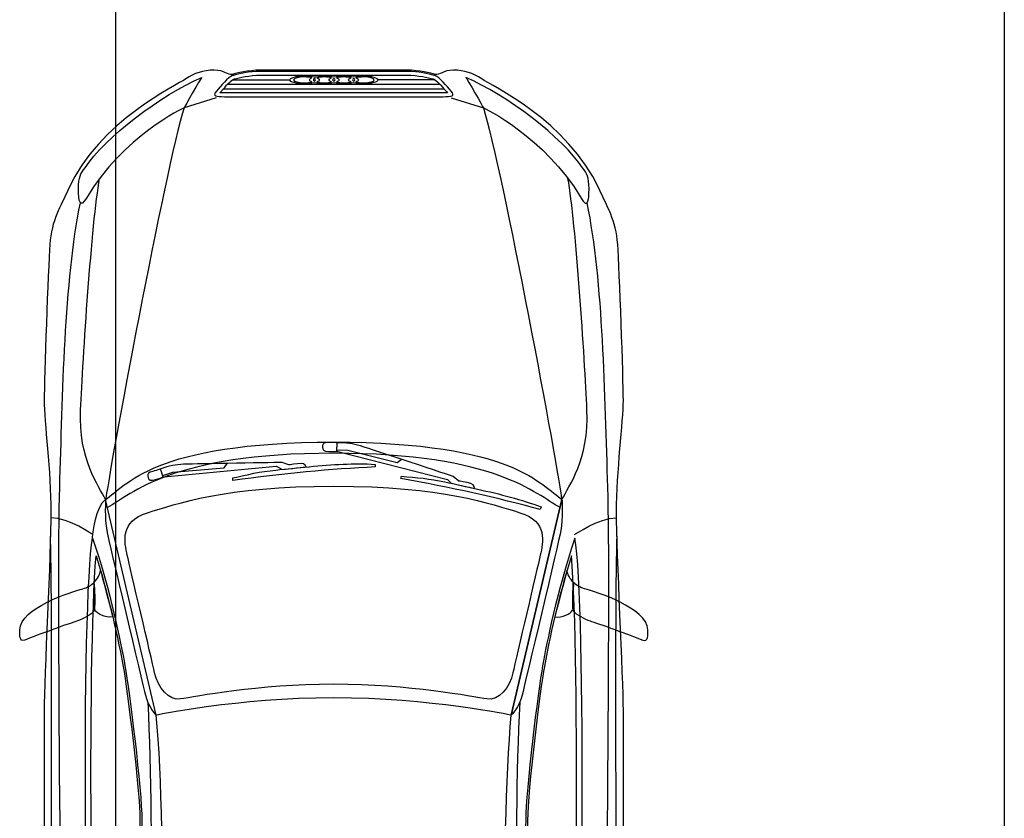
# Model space of a CAD drawing. Units: inches. Extents: x 1863 to 2938, y 1238 to 2492.
# Tile 4 of 12: x 2217 to 2283, y 1398 to 1452. Entities that reach past the tile are written whole.
import ezdxf

# ---------------------------------------------------------------- set-up
doc = ezdxf.new("R2010")
doc.units = ezdxf.units.IN
doc.layers.add('A-ANNO-DIMS', color=2, linetype='Continuous', lineweight=18)
doc.layers.add('AUDI', color=7, linetype='Continuous', lineweight=25)
doc.styles.get("Standard").update_dxf_attribs({"font": 'arial.ttf'})
doc.dimstyles.new('ISO-25', dxfattribs={"dimtxt": 7, "dimasz": 2.5, "dimexe": 1.25, "dimexo": 0.625, "dimtad": 1, "dimdec": 0, "dimlunit": 3, "dimtxsty": 'Standard', "dimcen": 2.5, "dimadec": 0, "dimazin": 0, "dimtfac": 1, "dimtdec": 0, "dimtmove": 0, "dimatfit": 3, "dimfxl": 1, "dimarcsym": 0})

# ---------------------------------------------------------------- blocks, each defined once
blk = doc.blocks.new('*D58')
at = {"layer": 'A-ANNO-DIMS', "color": 0, "lineweight": -2, "transparency": 16777216}
for p, q in [((2283.384, 1624.448), (2283.384, 1243.072)), ((2223.915, 1623.598), (2223.915, 1243.072)), ((2226.415, 1244.322), (2280.884, 1244.322))]:
    blk.add_line(p, q, dxfattribs=at)
at = {"layer": 'A-ANNO-DIMS', "color": 0, "transparency": 16777216}
for points in [[(2226.415, 1244.739), (2226.415, 1243.905), (2223.915, 1244.322)], [(2280.884, 1244.739), (2280.884, 1243.905), (2283.384, 1244.322)]]:
    blk.add_solid(points, dxfattribs=at)
at = {"layer": 'Defpoints', "color": 0, "transparency": 16777216}
for p in [(2283.384, 1625.073), (2223.915, 1624.223), (2283.384, 1244.322)]:
    blk.add_point(p, dxfattribs=at)
at = {"layer": 'A-ANNO-DIMS', "color": 0, "transparency": 16777216, "insert": (2253.65, 1248.566), "char_height": 7, "attachment_point": 5}
blk.add_mtext('4\'-11 1/2"', dxfattribs=at)

msp = doc.modelspace()

# ---------------------------------------------------------------- linework, layer by layer
at = {"layer": 'AUDI'}
for points, knots in [([(2238.512, 1351.601), (2224.304, 1351.757), (2222.24, 1356.535), (2221.369, 1359.683), (2221.369, 1359.683), (2220.8, 1361.542), (2220.345, 1363.021), (2220.118, 1363.779), (2220.118, 1363.779), (2219.89, 1364.538), (2219.398, 1366.852), (2219.359, 1368.786), (2219.359, 1368.786), (2219.321, 1370.721), (2219.134, 1382.255), (2219.134, 1385.438), (2219.134, 1385.438), (2219.134, 1388.621), (2219.134, 1403.534), (2219.134, 1405.655), (2219.134, 1405.655), (2219.134, 1407.776), (2219.587, 1416.238), (2219.587, 1418.931), (2219.587, 1418.931), (2219.587, 1421.624), (2219.134, 1425.003), (2219.134, 1426.403), (2219.134, 1426.403), (2219.134, 1427.803), (2219.397, 1435.203), (2219.511, 1436.834), (2219.511, 1436.834), (2219.625, 1438.465), (2220.236, 1439.39), (2220.762, 1440.551), (2220.762, 1440.551), (2222.809, 1445.064), (2228.041, 1447.53), (2228.61, 1447.909), (2228.61, 1447.909), (2229.178, 1448.289), (2229.782, 1448.495), (2230.505, 1448.495), (2230.505, 1448.495), (2231.228, 1448.495), (2231.415, 1448.137), (2231.718, 1448.213), (2231.718, 1448.213), (2232.021, 1448.289), (2232.777, 1448.495), (2233.614, 1448.495), (2233.614, 1448.495), (2234.451, 1448.495), (2238.512, 1448.495), (2238.512, 1448.495), (2238.512, 1448.495), (2238.512, 1448.495), (2242.574, 1448.495), (2243.411, 1448.495), (2243.411, 1448.495), (2244.248, 1448.495), (2245.003, 1448.289), (2245.306, 1448.213), (2245.306, 1448.213), (2245.61, 1448.137), (2245.796, 1448.495), (2246.52, 1448.495), (2246.52, 1448.495), (2247.243, 1448.495), (2247.846, 1448.289), (2248.415, 1447.909), (2248.415, 1447.909), (2248.984, 1447.53), (2254.215, 1445.064), (2256.262, 1440.551), (2256.262, 1440.551), (2256.789, 1439.39), (2257.4, 1438.465), (2257.513, 1436.834), (2257.513, 1436.834), (2257.627, 1435.203), (2257.891, 1427.803), (2257.891, 1426.403), (2257.891, 1426.403), (2257.891, 1425.003), (2257.438, 1421.624), (2257.438, 1418.931), (2257.438, 1418.931), (2257.438, 1416.238), (2257.891, 1407.776), (2257.891, 1405.655), (2257.891, 1405.655), (2257.891, 1403.534), (2257.891, 1388.621), (2257.891, 1385.438), (2257.891, 1385.438), (2257.891, 1382.255), (2257.703, 1370.721), (2257.665, 1368.786), (2257.665, 1368.786), (2257.627, 1366.852), (2257.134, 1364.538), (2256.907, 1363.779), (2256.907, 1363.779), (2256.679, 1363.021), (2256.225, 1361.541), (2255.656, 1359.683), (2255.656, 1359.683), (2254.784, 1356.535), (2252.721, 1351.757), (2238.512, 1351.601)], [0, 0, 0, 0, 0.035714, 0.035714, 0.035714, 0.035714, 0.071429, 0.071429, 0.071429, 0.071429, 0.107143, 0.107143, 0.107143, 0.107143, 0.142857, 0.142857, 0.142857, 0.142857, 0.178571, 0.178571, 0.178571, 0.178571, 0.214286, 0.214286, 0.214286, 0.214286, 0.25, 0.25, 0.25, 0.25, 0.285714, 0.285714, 0.285714, 0.285714, 0.321429, 0.321429, 0.321429, 0.321429, 0.357143, 0.357143, 0.357143, 0.357143, 0.392857, 0.392857, 0.392857, 0.392857, 0.428571, 0.428571, 0.428571, 0.428571, 0.464286, 0.464286, 0.464286, 0.464286, 0.5, 0.5, 0.5, 0.5, 0.535714, 0.535714, 0.535714, 0.535714, 0.571429, 0.571429, 0.571429, 0.571429, 0.607143, 0.607143, 0.607143, 0.607143, 0.642857, 0.642857, 0.642857, 0.642857, 0.678571, 0.678571, 0.678571, 0.678571, 0.714286, 0.714286, 0.714286, 0.714286, 0.75, 0.75, 0.75, 0.75, 0.785714, 0.785714, 0.785714, 0.785714, 0.821429, 0.821429, 0.821429, 0.821429, 0.857143, 0.857143, 0.857143, 0.857143, 0.892857, 0.892857, 0.892857, 0.892857, 0.928571, 0.928571, 0.928571, 0.928571, 0.964286, 0.964286, 0.964286, 0.964286, 1, 1, 1, 1]), ([(2238.592, 1448.412), (2238.592, 1448.412), (2243.411, 1448.412), (2243.411, 1448.412), (2243.411, 1448.412), (2244.184, 1448.412), (2244.885, 1448.234), (2245.222, 1448.149), (2245.222, 1448.149), (2245.222, 1448.149), (2245.286, 1448.132), (2245.286, 1448.132), (2245.286, 1448.132), (2245.593, 1448.035), (2246.067, 1447.418), (2246.367, 1447.086), (2246.367, 1447.086), (2246.667, 1446.754), (2246.367, 1446.722), (2245.83, 1446.722), (2245.83, 1446.722), (2245.292, 1446.722), (2238.512, 1446.722), (2238.512, 1446.722), (2238.512, 1446.722), (2238.512, 1446.722), (2231.732, 1446.722), (2231.195, 1446.722), (2231.195, 1446.722), (2230.658, 1446.722), (2230.357, 1446.754), (2230.658, 1447.086), (2230.658, 1447.086), (2230.958, 1447.418), (2231.432, 1448.034), (2231.738, 1448.132), (2231.738, 1448.132), (2231.738, 1448.132), (2231.802, 1448.149), (2231.802, 1448.149), (2231.802, 1448.149), (2232.139, 1448.234), (2232.841, 1448.412), (2233.614, 1448.412), (2233.614, 1448.412), (2233.614, 1448.412), (2238.433, 1448.412), (2238.433, 1448.412), (2238.433, 1448.412), (2238.433, 1448.412), (2238.592, 1448.412), (2238.592, 1448.412)], [0, 0, 0, 0, 0.076923, 0.076923, 0.076923, 0.076923, 0.153846, 0.153846, 0.153846, 0.153846, 0.230769, 0.230769, 0.230769, 0.230769, 0.307692, 0.307692, 0.307692, 0.307692, 0.384615, 0.384615, 0.384615, 0.384615, 0.461538, 0.461538, 0.461538, 0.461538, 0.538462, 0.538462, 0.538462, 0.538462, 0.615385, 0.615385, 0.615385, 0.615385, 0.692308, 0.692308, 0.692308, 0.692308, 0.769231, 0.769231, 0.769231, 0.769231, 0.846154, 0.846154, 0.846154, 0.846154, 0.923077, 0.923077, 0.923077, 0.923077, 1, 1, 1, 1]), ([(2221.431, 1440.56), (2221.431, 1439.717), (2221.527, 1439.205), (2221.96, 1439.937), (2221.96, 1439.937), (2224.389, 1444.05), (2228.5, 1445.982), (2228.5, 1445.982), (2228.5, 1445.982), (2228.5, 1445.982), (2229.614, 1447.98), (2229.684, 1448.008), (2229.684, 1448.008), (2226.972, 1446.86), (2223.162, 1443.967), (2221.867, 1441.963), (2221.867, 1441.963), (2221.555, 1441.557), (2221.431, 1441.355), (2221.431, 1440.56)], [0, 0, 0, 0, 0.2, 0.2, 0.2, 0.2, 0.4, 0.4, 0.4, 0.4, 0.6, 0.6, 0.6, 0.6, 0.8, 0.8, 0.8, 0.8, 1, 1, 1, 1]), ([(2221.431, 1440.56), (2221.431, 1439.717), (2221.527, 1439.205), (2221.96, 1439.937), (2221.96, 1439.937), (2224.389, 1444.05), (2228.5, 1445.982), (2228.5, 1445.982), (2228.5, 1445.982), (2228.5, 1445.982), (2229.614, 1447.98), (2229.684, 1448.008), (2229.684, 1448.008), (2226.972, 1446.86), (2223.162, 1443.967), (2221.867, 1441.963), (2221.867, 1441.963), (2221.555, 1441.557), (2221.431, 1441.355), (2221.431, 1440.56)], [0, 0, 0, 0, 0.2, 0.2, 0.2, 0.2, 0.4, 0.4, 0.4, 0.4, 0.6, 0.6, 0.6, 0.6, 0.8, 0.8, 0.8, 0.8, 1, 1, 1, 1]), ([(2231.195, 1446.973), (2231.195, 1446.973), (2231.195, 1446.973), (2231.195, 1446.973), (2231.195, 1446.973), (2231.195, 1446.973), (2245.83, 1446.973), (2245.83, 1446.973), (2245.83, 1446.973), (2245.953, 1446.973), (2246.048, 1446.976), (2246.125, 1446.981), (2246.125, 1446.981), (2246.066, 1447.049), (2245.975, 1447.153), (2245.975, 1447.153), (2245.975, 1447.153), (2245.755, 1447.409), (2245.387, 1447.836), (2245.21, 1447.893), (2245.21, 1447.893), (2245.21, 1447.893), (2245.161, 1447.905), (2245.161, 1447.905), (2245.161, 1447.905), (2244.832, 1447.988), (2244.152, 1448.161), (2243.411, 1448.161), (2243.411, 1448.161), (2243.411, 1448.161), (2233.614, 1448.161), (2233.614, 1448.161), (2233.614, 1448.161), (2232.873, 1448.161), (2232.192, 1447.988), (2231.865, 1447.906), (2231.865, 1447.906), (2231.865, 1447.906), (2231.8, 1447.889), (2231.8, 1447.889), (2231.8, 1447.889), (2231.638, 1447.837), (2231.27, 1447.409), (2231.05, 1447.153), (2231.05, 1447.153), (2231.05, 1447.153), (2230.959, 1447.049), (2230.899, 1446.981), (2230.899, 1446.981), (2230.976, 1446.976), (2231.071, 1446.973), (2231.195, 1446.973)], [0, 0, 0, 0, 0.076923, 0.076923, 0.076923, 0.076923, 0.153846, 0.153846, 0.153846, 0.153846, 0.230769, 0.230769, 0.230769, 0.230769, 0.307692, 0.307692, 0.307692, 0.307692, 0.384615, 0.384615, 0.384615, 0.384615, 0.461538, 0.461538, 0.461538, 0.461538, 0.538462, 0.538462, 0.538462, 0.538462, 0.615385, 0.615385, 0.615385, 0.615385, 0.692308, 0.692308, 0.692308, 0.692308, 0.769231, 0.769231, 0.769231, 0.769231, 0.846154, 0.846154, 0.846154, 0.846154, 0.923077, 0.923077, 0.923077, 0.923077, 1, 1, 1, 1]), ([(2236.558, 1447.584), (2236.813, 1447.584), (2237.036, 1447.61), (2237.211, 1447.653), (2237.211, 1447.653), (2237.386, 1447.61), (2237.625, 1447.584), (2237.88, 1447.584), (2237.88, 1447.584), (2238.135, 1447.584), (2238.358, 1447.61), (2238.533, 1447.649), (2238.533, 1447.649), (2238.692, 1447.61), (2238.932, 1447.584), (2239.17, 1447.584), (2239.17, 1447.584), (2239.425, 1447.584), (2239.664, 1447.61), (2239.84, 1447.653), (2239.84, 1447.653), (2240.015, 1447.61), (2240.238, 1447.584), (2240.492, 1447.584), (2240.492, 1447.584), (2241.034, 1447.584), (2241.48, 1447.7), (2241.48, 1447.846), (2241.48, 1447.846), (2241.48, 1447.988), (2241.034, 1448.108), (2240.492, 1448.108), (2240.492, 1448.108), (2240.238, 1448.108), (2240.015, 1448.078), (2239.84, 1448.039), (2239.84, 1448.039), (2239.664, 1448.078), (2239.425, 1448.108), (2239.17, 1448.108), (2239.17, 1448.108), (2238.932, 1448.108), (2238.692, 1448.082), (2238.533, 1448.039), (2238.533, 1448.039), (2238.358, 1448.082), (2238.135, 1448.108), (2237.88, 1448.108), (2237.88, 1448.108), (2237.596, 1448.108), (2237.289, 1448.057), (2237.211, 1448.039), (2237.211, 1448.039), (2237.036, 1448.078), (2236.813, 1448.108), (2236.558, 1448.108), (2236.558, 1448.108), (2236.016, 1448.108), (2235.57, 1447.988), (2235.57, 1447.846), (2235.57, 1447.846), (2235.57, 1447.7), (2236.016, 1447.584), (2236.558, 1447.584)], [0, 0, 0, 0, 0.0625, 0.0625, 0.0625, 0.0625, 0.125, 0.125, 0.125, 0.125, 0.1875, 0.1875, 0.1875, 0.1875, 0.25, 0.25, 0.25, 0.25, 0.3125, 0.3125, 0.3125, 0.3125, 0.375, 0.375, 0.375, 0.375, 0.4375, 0.4375, 0.4375, 0.4375, 0.5, 0.5, 0.5, 0.5, 0.5625, 0.5625, 0.5625, 0.5625, 0.625, 0.625, 0.625, 0.625, 0.6875, 0.6875, 0.6875, 0.6875, 0.75, 0.75, 0.75, 0.75, 0.8125, 0.8125, 0.8125, 0.8125, 0.875, 0.875, 0.875, 0.875, 0.9375, 0.9375, 0.9375, 0.9375, 1, 1, 1, 1]), ([(2236.558, 1447.584), (2236.813, 1447.584), (2237.036, 1447.61), (2237.211, 1447.653), (2237.211, 1447.653), (2237.386, 1447.61), (2237.625, 1447.584), (2237.88, 1447.584), (2237.88, 1447.584), (2238.135, 1447.584), (2238.358, 1447.61), (2238.533, 1447.649), (2238.533, 1447.649), (2238.692, 1447.61), (2238.932, 1447.584), (2239.17, 1447.584), (2239.17, 1447.584), (2239.425, 1447.584), (2239.664, 1447.61), (2239.84, 1447.653), (2239.84, 1447.653), (2240.015, 1447.61), (2240.238, 1447.584), (2240.492, 1447.584), (2240.492, 1447.584), (2241.034, 1447.584), (2241.48, 1447.7), (2241.48, 1447.846), (2241.48, 1447.846), (2241.48, 1447.988), (2241.034, 1448.108), (2240.492, 1448.108), (2240.492, 1448.108), (2240.238, 1448.108), (2240.015, 1448.078), (2239.84, 1448.039), (2239.84, 1448.039), (2239.664, 1448.078), (2239.425, 1448.108), (2239.17, 1448.108), (2239.17, 1448.108), (2238.932, 1448.108), (2238.692, 1448.082), (2238.533, 1448.039), (2238.533, 1448.039), (2238.358, 1448.082), (2238.135, 1448.108), (2237.88, 1448.108), (2237.88, 1448.108), (2237.596, 1448.108), (2237.289, 1448.057), (2237.211, 1448.039), (2237.211, 1448.039), (2237.036, 1448.078), (2236.813, 1448.108), (2236.558, 1448.108), (2236.558, 1448.108), (2236.016, 1448.108), (2235.57, 1447.988), (2235.57, 1447.846), (2235.57, 1447.846), (2235.57, 1447.7), (2236.016, 1447.584), (2236.558, 1447.584)], [0, 0, 0, 0, 0.0625, 0.0625, 0.0625, 0.0625, 0.125, 0.125, 0.125, 0.125, 0.1875, 0.1875, 0.1875, 0.1875, 0.25, 0.25, 0.25, 0.25, 0.3125, 0.3125, 0.3125, 0.3125, 0.375, 0.375, 0.375, 0.375, 0.4375, 0.4375, 0.4375, 0.4375, 0.5, 0.5, 0.5, 0.5, 0.5625, 0.5625, 0.5625, 0.5625, 0.625, 0.625, 0.625, 0.625, 0.6875, 0.6875, 0.6875, 0.6875, 0.75, 0.75, 0.75, 0.75, 0.8125, 0.8125, 0.8125, 0.8125, 0.875, 0.875, 0.875, 0.875, 0.9375, 0.9375, 0.9375, 0.9375, 1, 1, 1, 1]), ([(2236.558, 1448.039), (2236.749, 1448.039), (2236.925, 1448.022), (2237.052, 1447.988), (2237.052, 1447.988), (2236.956, 1447.945), (2236.892, 1447.898), (2236.892, 1447.846), (2236.892, 1447.846), (2236.892, 1447.79), (2236.956, 1447.743), (2237.052, 1447.7), (2237.052, 1447.7), (2236.925, 1447.67), (2236.749, 1447.649), (2236.558, 1447.649), (2236.558, 1447.649), (2236.144, 1447.649), (2235.825, 1447.735), (2235.825, 1447.846), (2235.825, 1447.846), (2235.825, 1447.953), (2236.144, 1448.039), (2236.558, 1448.039)], [0, 0, 0, 0, 0.166667, 0.166667, 0.166667, 0.166667, 0.333333, 0.333333, 0.333333, 0.333333, 0.5, 0.5, 0.5, 0.5, 0.666667, 0.666667, 0.666667, 0.666667, 0.833333, 0.833333, 0.833333, 0.833333, 1, 1, 1, 1]), ([(2237.291, 1447.846), (2237.291, 1447.812), (2237.259, 1447.786), (2237.211, 1447.76), (2237.211, 1447.76), (2237.163, 1447.786), (2237.147, 1447.812), (2237.147, 1447.846), (2237.147, 1447.846), (2237.147, 1447.876), (2237.163, 1447.906), (2237.211, 1447.932), (2237.211, 1447.932), (2237.259, 1447.906), (2237.291, 1447.876), (2237.291, 1447.846)], [0, 0, 0, 0, 0.25, 0.25, 0.25, 0.25, 0.5, 0.5, 0.5, 0.5, 0.75, 0.75, 0.75, 0.75, 1, 1, 1, 1]), ([(2238.358, 1447.992), (2238.262, 1447.949), (2238.199, 1447.898), (2238.199, 1447.846), (2238.199, 1447.846), (2238.199, 1447.79), (2238.262, 1447.739), (2238.358, 1447.696), (2238.358, 1447.696), (2238.231, 1447.666), (2238.071, 1447.649), (2237.88, 1447.649), (2237.88, 1447.649), (2237.689, 1447.649), (2237.514, 1447.67), (2237.386, 1447.7), (2237.386, 1447.7), (2237.482, 1447.743), (2237.546, 1447.79), (2237.546, 1447.846), (2237.546, 1447.846), (2237.546, 1447.898), (2237.482, 1447.945), (2237.386, 1447.988), (2237.386, 1447.988), (2237.514, 1448.022), (2237.689, 1448.039), (2237.88, 1448.039), (2237.88, 1448.039), (2238.071, 1448.039), (2238.231, 1448.022), (2238.358, 1447.992)], [0, 0, 0, 0, 0.125, 0.125, 0.125, 0.125, 0.25, 0.25, 0.25, 0.25, 0.375, 0.375, 0.375, 0.375, 0.5, 0.5, 0.5, 0.5, 0.625, 0.625, 0.625, 0.625, 0.75, 0.75, 0.75, 0.75, 0.875, 0.875, 0.875, 0.875, 1, 1, 1, 1]), ([(2238.613, 1447.846), (2238.613, 1447.812), (2238.581, 1447.782), (2238.533, 1447.752), (2238.533, 1447.752), (2238.469, 1447.782), (2238.438, 1447.812), (2238.438, 1447.846), (2238.438, 1447.846), (2238.438, 1447.876), (2238.469, 1447.91), (2238.533, 1447.936), (2238.533, 1447.936), (2238.581, 1447.911), (2238.613, 1447.876), (2238.613, 1447.846)], [0, 0, 0, 0, 0.25, 0.25, 0.25, 0.25, 0.5, 0.5, 0.5, 0.5, 0.75, 0.75, 0.75, 0.75, 1, 1, 1, 1]), ([(2239.68, 1447.988), (2239.569, 1447.945), (2239.505, 1447.898), (2239.505, 1447.846), (2239.505, 1447.846), (2239.505, 1447.79), (2239.569, 1447.743), (2239.68, 1447.7), (2239.68, 1447.7), (2239.537, 1447.67), (2239.362, 1447.649), (2239.17, 1447.649), (2239.17, 1447.649), (2238.995, 1447.649), (2238.82, 1447.666), (2238.692, 1447.696), (2238.692, 1447.696), (2238.804, 1447.739), (2238.868, 1447.79), (2238.868, 1447.846), (2238.868, 1447.846), (2238.868, 1447.898), (2238.804, 1447.949), (2238.692, 1447.992), (2238.692, 1447.992), (2238.82, 1448.022), (2238.995, 1448.039), (2239.17, 1448.039), (2239.17, 1448.039), (2239.362, 1448.039), (2239.537, 1448.022), (2239.68, 1447.988)], [0, 0, 0, 0, 0.125, 0.125, 0.125, 0.125, 0.25, 0.25, 0.25, 0.25, 0.375, 0.375, 0.375, 0.375, 0.5, 0.5, 0.5, 0.5, 0.625, 0.625, 0.625, 0.625, 0.75, 0.75, 0.75, 0.75, 0.875, 0.875, 0.875, 0.875, 1, 1, 1, 1]), ([(2239.919, 1447.846), (2239.919, 1447.812), (2239.887, 1447.786), (2239.84, 1447.76), (2239.84, 1447.76), (2239.792, 1447.786), (2239.76, 1447.812), (2239.76, 1447.846), (2239.76, 1447.846), (2239.76, 1447.876), (2239.792, 1447.906), (2239.84, 1447.932), (2239.84, 1447.932), (2239.887, 1447.906), (2239.919, 1447.876), (2239.919, 1447.846)], [0, 0, 0, 0, 0.25, 0.25, 0.25, 0.25, 0.5, 0.5, 0.5, 0.5, 0.75, 0.75, 0.75, 0.75, 1, 1, 1, 1]), ([(2241.225, 1447.846), (2241.225, 1447.735), (2240.907, 1447.649), (2240.492, 1447.649), (2240.492, 1447.649), (2240.301, 1447.649), (2240.126, 1447.67), (2239.999, 1447.7), (2239.999, 1447.7), (2240.094, 1447.743), (2240.158, 1447.79), (2240.158, 1447.846), (2240.158, 1447.846), (2240.158, 1447.898), (2240.094, 1447.945), (2239.999, 1447.988), (2239.999, 1447.988), (2240.126, 1448.022), (2240.301, 1448.039), (2240.492, 1448.039), (2240.492, 1448.039), (2240.907, 1448.039), (2241.225, 1447.953), (2241.225, 1447.846)], [0, 0, 0, 0, 0.166667, 0.166667, 0.166667, 0.166667, 0.333333, 0.333333, 0.333333, 0.333333, 0.5, 0.5, 0.5, 0.5, 0.666667, 0.666667, 0.666667, 0.666667, 0.833333, 0.833333, 0.833333, 0.833333, 1, 1, 1, 1]), ([(2255.594, 1440.56), (2255.594, 1439.717), (2255.497, 1439.205), (2255.065, 1439.937), (2255.065, 1439.937), (2252.635, 1444.05), (2248.524, 1445.982), (2248.524, 1445.982), (2248.524, 1445.982), (2248.524, 1445.982), (2247.41, 1447.98), (2247.341, 1448.008), (2247.341, 1448.008), (2250.053, 1446.86), (2253.862, 1443.967), (2255.158, 1441.963), (2255.158, 1441.963), (2255.469, 1441.557), (2255.594, 1441.355), (2255.594, 1440.56)], [0, 0, 0, 0, 0.2, 0.2, 0.2, 0.2, 0.4, 0.4, 0.4, 0.4, 0.6, 0.6, 0.6, 0.6, 0.8, 0.8, 0.8, 0.8, 1, 1, 1, 1]), ([(2255.594, 1440.56), (2255.594, 1439.717), (2255.497, 1439.205), (2255.065, 1439.937), (2255.065, 1439.937), (2252.635, 1444.05), (2248.524, 1445.982), (2248.524, 1445.982), (2248.524, 1445.982), (2248.524, 1445.982), (2247.41, 1447.98), (2247.341, 1448.008), (2247.341, 1448.008), (2250.053, 1446.86), (2253.862, 1443.967), (2255.158, 1441.963), (2255.158, 1441.963), (2255.469, 1441.557), (2255.594, 1441.355), (2255.594, 1440.56)], [0, 0, 0, 0, 0.2, 0.2, 0.2, 0.2, 0.4, 0.4, 0.4, 0.4, 0.6, 0.6, 0.6, 0.6, 0.8, 0.8, 0.8, 0.8, 1, 1, 1, 1]), ([(2223.24, 1419.775), (2222.797, 1420.661), (2221.424, 1422.428), (2221.571, 1425.767), (2221.571, 1425.767), (2221.717, 1429.106), (2222.31, 1438.318), (2222.842, 1441.249)], [0, 0, 0, 0, 0.5, 0.5, 0.5, 0.5, 1, 1, 1, 1]), ([(2253.785, 1419.775), (2254.227, 1420.661), (2255.6, 1422.428), (2255.454, 1425.767), (2255.454, 1425.767), (2255.308, 1429.106), (2254.715, 1438.318), (2254.183, 1441.249)], [0, 0, 0, 0, 0.5, 0.5, 0.5, 0.5, 1, 1, 1, 1]), ([(2222.035, 1359.641), (2221.321, 1363.213), (2220.561, 1370.446), (2220.431, 1377.979), (2220.431, 1377.979), (2220.301, 1385.512), (2219.977, 1414.474), (2220.172, 1420.578), (2220.172, 1420.578), (2220.366, 1426.682), (2220.475, 1434.382), (2221.557, 1439.624)], [0, 0, 0, 0, 0.333333, 0.333333, 0.333333, 0.333333, 0.666667, 0.666667, 0.666667, 0.666667, 1, 1, 1, 1]), ([(2254.99, 1359.641), (2255.704, 1363.213), (2256.464, 1370.446), (2256.593, 1377.979), (2256.593, 1377.979), (2256.723, 1385.512), (2257.048, 1414.474), (2256.853, 1420.578), (2256.853, 1420.578), (2256.658, 1426.682), (2256.549, 1434.382), (2255.468, 1439.624)], [0, 0, 0, 0, 0.333333, 0.333333, 0.333333, 0.333333, 0.666667, 0.666667, 0.666667, 0.666667, 1, 1, 1, 1]), ([(2238.512, 1406.494), (2244.944, 1406.494), (2250.394, 1405.331), (2250.394, 1405.331), (2250.394, 1405.331), (2250.394, 1405.331), (2253.785, 1419.775), (2253.785, 1419.775), (2253.785, 1419.775), (2252.428, 1420.648), (2250.661, 1423.605), (2238.512, 1423.605), (2238.512, 1423.605), (2226.364, 1423.605), (2224.596, 1420.648), (2223.24, 1419.775), (2223.24, 1419.775), (2223.24, 1419.775), (2226.631, 1405.331), (2226.631, 1405.331), (2226.631, 1405.331), (2226.631, 1405.331), (2232.081, 1406.494), (2238.512, 1406.494)], [0, 0, 0, 0, 0.166667, 0.166667, 0.166667, 0.166667, 0.333333, 0.333333, 0.333333, 0.333333, 0.5, 0.5, 0.5, 0.5, 0.666667, 0.666667, 0.666667, 0.666667, 0.833333, 0.833333, 0.833333, 0.833333, 1, 1, 1, 1]), ([(2238.512, 1406.494), (2244.944, 1406.494), (2250.394, 1405.331), (2250.394, 1405.331), (2250.394, 1405.331), (2250.394, 1405.331), (2253.785, 1419.775), (2253.785, 1419.775), (2253.785, 1419.775), (2252.428, 1420.648), (2250.661, 1423.605), (2238.512, 1423.605), (2238.512, 1423.605), (2226.364, 1423.605), (2224.596, 1420.648), (2223.24, 1419.775), (2223.24, 1419.775), (2223.24, 1419.775), (2226.631, 1405.331), (2226.631, 1405.331), (2226.631, 1405.331), (2226.631, 1405.331), (2232.081, 1406.494), (2238.512, 1406.494)], [0, 0, 0, 0, 0.166667, 0.166667, 0.166667, 0.166667, 0.333333, 0.333333, 0.333333, 0.333333, 0.5, 0.5, 0.5, 0.5, 0.666667, 0.666667, 0.666667, 0.666667, 0.833333, 0.833333, 0.833333, 0.833333, 1, 1, 1, 1]), ([(2238.952, 1423.555), (2239.542, 1423.555), (2239.972, 1423.459), (2240.482, 1423.299), (2240.482, 1423.299), (2240.864, 1423.188), (2246.503, 1421.307), (2246.503, 1421.307), (2246.503, 1421.307), (2246.503, 1421.307), (2246.885, 1421.004), (2246.885, 1421.004), (2246.885, 1421.004), (2246.885, 1421.004), (2247.395, 1420.909), (2247.682, 1420.845), (2247.682, 1420.845), (2247.968, 1420.766), (2247.936, 1420.51), (2247.936, 1420.51), (2247.936, 1420.51), (2247.936, 1420.51), (2246.375, 1420.861), (2246.375, 1420.861), (2246.375, 1420.861), (2246.375, 1420.861), (2246.121, 1421.116), (2246.121, 1421.116), (2246.121, 1421.116), (2246.121, 1421.116), (2238.793, 1422.981), (2238.793, 1422.981), (2238.793, 1422.981), (2238.793, 1422.981), (2238.554, 1422.981), (2238.188, 1422.981), (2238.188, 1422.981), (2237.821, 1422.997), (2237.758, 1423.124), (2237.758, 1423.267), (2237.758, 1423.267), (2237.758, 1423.427), (2237.774, 1423.571), (2237.997, 1423.571), (2237.997, 1423.571), (2238.22, 1423.586), (2238.586, 1423.571), (2238.952, 1423.555)], [0, 0, 0, 0, 0.083333, 0.083333, 0.083333, 0.083333, 0.166667, 0.166667, 0.166667, 0.166667, 0.25, 0.25, 0.25, 0.25, 0.333333, 0.333333, 0.333333, 0.333333, 0.416667, 0.416667, 0.416667, 0.416667, 0.5, 0.5, 0.5, 0.5, 0.583333, 0.583333, 0.583333, 0.583333, 0.666667, 0.666667, 0.666667, 0.666667, 0.75, 0.75, 0.75, 0.75, 0.833333, 0.833333, 0.833333, 0.833333, 0.916667, 0.916667, 0.916667, 0.916667, 1, 1, 1, 1]), ([(2253.657, 1419.23), (2252.005, 1420.108), (2249.453, 1422.859), (2238.512, 1422.859), (2238.512, 1422.859), (2227.572, 1422.859), (2225.02, 1420.108), (2223.368, 1419.23)], [0, 0, 0, 0, 0.5, 0.5, 0.5, 0.5, 1, 1, 1, 1]), ([(2238.713, 1423.092), (2238.713, 1423.092), (2239.446, 1423.076), (2239.446, 1423.076), (2239.446, 1423.076), (2239.446, 1423.076), (2242.759, 1422.247), (2242.759, 1422.247), (2242.759, 1422.247), (2242.759, 1422.247), (2243.03, 1422.455), (2243.03, 1422.455)], [0, 0, 0, 0, 0.333333, 0.333333, 0.333333, 0.333333, 0.666667, 0.666667, 0.666667, 0.666667, 1, 1, 1, 1]), ([(2227.133, 1421.881), (2227.674, 1422.072), (2228.12, 1422.12), (2228.662, 1422.136), (2228.662, 1422.136), (2229.06, 1422.136), (2235.05, 1422.247), (2235.05, 1422.247), (2235.05, 1422.247), (2235.05, 1422.247), (2235.511, 1422.088), (2235.511, 1422.088), (2235.511, 1422.088), (2235.511, 1422.088), (2236.037, 1422.152), (2236.324, 1422.168), (2236.324, 1422.168), (2236.611, 1422.2), (2236.658, 1421.945), (2236.658, 1421.945), (2236.658, 1421.945), (2236.658, 1421.945), (2235.082, 1421.785), (2235.082, 1421.785), (2235.082, 1421.785), (2235.082, 1421.785), (2234.651, 1421.992), (2234.651, 1421.992), (2234.651, 1421.992), (2234.651, 1421.992), (2227.165, 1421.291), (2227.165, 1421.291), (2227.165, 1421.291), (2227.165, 1421.291), (2226.942, 1421.212), (2226.591, 1421.1), (2226.591, 1421.1), (2226.256, 1420.989), (2226.145, 1421.084), (2226.097, 1421.228), (2226.097, 1421.228), (2226.049, 1421.387), (2226.018, 1421.515), (2226.225, 1421.594), (2226.225, 1421.594), (2226.432, 1421.658), (2226.782, 1421.769), (2227.133, 1421.881)], [0, 0, 0, 0, 0.083333, 0.083333, 0.083333, 0.083333, 0.166667, 0.166667, 0.166667, 0.166667, 0.25, 0.25, 0.25, 0.25, 0.333333, 0.333333, 0.333333, 0.333333, 0.416667, 0.416667, 0.416667, 0.416667, 0.5, 0.5, 0.5, 0.5, 0.583333, 0.583333, 0.583333, 0.583333, 0.666667, 0.666667, 0.666667, 0.666667, 0.75, 0.75, 0.75, 0.75, 0.833333, 0.833333, 0.833333, 0.833333, 0.916667, 0.916667, 0.916667, 0.916667, 1, 1, 1, 1]), ([(2227.133, 1421.881), (2227.674, 1422.072), (2228.12, 1422.12), (2228.662, 1422.136), (2228.662, 1422.136), (2229.06, 1422.136), (2235.05, 1422.247), (2235.05, 1422.247), (2235.05, 1422.247), (2235.05, 1422.247), (2235.511, 1422.088), (2235.511, 1422.088), (2235.511, 1422.088), (2235.511, 1422.088), (2236.037, 1422.152), (2236.324, 1422.168), (2236.324, 1422.168), (2236.611, 1422.2), (2236.658, 1421.945), (2236.658, 1421.945), (2236.658, 1421.945), (2236.658, 1421.945), (2235.082, 1421.785), (2235.082, 1421.785), (2235.082, 1421.785), (2235.082, 1421.785), (2234.651, 1421.992), (2234.651, 1421.992), (2234.651, 1421.992), (2234.651, 1421.992), (2227.165, 1421.291), (2227.165, 1421.291), (2227.165, 1421.291), (2227.165, 1421.291), (2226.942, 1421.212), (2226.591, 1421.1), (2226.591, 1421.1), (2226.256, 1420.989), (2226.145, 1421.084), (2226.097, 1421.228), (2226.097, 1421.228), (2226.049, 1421.387), (2226.018, 1421.515), (2226.225, 1421.594), (2226.225, 1421.594), (2226.432, 1421.658), (2226.782, 1421.769), (2227.133, 1421.881)], [0, 0, 0, 0, 0.083333, 0.083333, 0.083333, 0.083333, 0.166667, 0.166667, 0.166667, 0.166667, 0.25, 0.25, 0.25, 0.25, 0.333333, 0.333333, 0.333333, 0.333333, 0.416667, 0.416667, 0.416667, 0.416667, 0.5, 0.5, 0.5, 0.5, 0.583333, 0.583333, 0.583333, 0.583333, 0.666667, 0.666667, 0.666667, 0.666667, 0.75, 0.75, 0.75, 0.75, 0.833333, 0.833333, 0.833333, 0.833333, 0.916667, 0.916667, 0.916667, 0.916667, 1, 1, 1, 1]), ([(2227.069, 1421.371), (2227.069, 1421.371), (2227.754, 1421.594), (2227.754, 1421.594), (2227.754, 1421.594), (2227.754, 1421.594), (2231.179, 1421.897), (2231.179, 1421.897), (2231.179, 1421.897), (2231.179, 1421.897), (2231.37, 1422.168), (2231.37, 1422.168)], [0, 0, 0, 0, 0.333333, 0.333333, 0.333333, 0.333333, 0.666667, 0.666667, 0.666667, 0.666667, 1, 1, 1, 1]), ([(2241.278, 1422.12), (2239.908, 1422.216), (2238.411, 1422.104), (2236.865, 1421.961), (2236.865, 1421.961), (2236.117, 1421.881), (2235.368, 1421.817), (2234.635, 1421.737), (2234.635, 1421.737), (2233.6, 1421.642), (2232.724, 1421.435), (2231.768, 1421.212), (2231.768, 1421.212), (2231.768, 1421.212), (2231.768, 1421.036), (2231.768, 1421.036), (2231.768, 1421.036), (2235.018, 1421.499), (2238.395, 1421.817), (2241.294, 1421.945), (2241.294, 1421.945), (2241.294, 1421.945), (2241.278, 1422.12), (2241.278, 1422.12)], [0, 0, 0, 0, 0.166667, 0.166667, 0.166667, 0.166667, 0.333333, 0.333333, 0.333333, 0.333333, 0.5, 0.5, 0.5, 0.5, 0.666667, 0.666667, 0.666667, 0.666667, 0.833333, 0.833333, 0.833333, 0.833333, 1, 1, 1, 1]), ([(2252.381, 1419.267), (2251.106, 1419.761), (2249.657, 1420.128), (2248.128, 1420.462), (2248.128, 1420.462), (2247.395, 1420.622), (2246.662, 1420.797), (2245.945, 1420.94), (2245.945, 1420.94), (2244.942, 1421.164), (2244.034, 1421.243), (2243.046, 1421.323), (2243.046, 1421.323), (2243.046, 1421.323), (2242.998, 1421.164), (2242.998, 1421.164), (2242.998, 1421.164), (2246.232, 1420.606), (2249.529, 1419.873), (2252.333, 1419.092), (2252.333, 1419.092), (2252.333, 1419.092), (2252.381, 1419.267), (2252.381, 1419.267)], [0, 0, 0, 0, 0.166667, 0.166667, 0.166667, 0.166667, 0.333333, 0.333333, 0.333333, 0.333333, 0.5, 0.5, 0.5, 0.5, 0.666667, 0.666667, 0.666667, 0.666667, 0.833333, 0.833333, 0.833333, 0.833333, 1, 1, 1, 1]), ([(2238.512, 1407.403), (2243.617, 1407.403), (2247.796, 1406.566), (2248.763, 1406.42), (2248.763, 1406.42), (2249.553, 1406.3), (2250.282, 1407.154), (2250.504, 1408.178), (2250.504, 1408.178), (2250.725, 1409.202), (2252.135, 1415.178), (2252.329, 1416.036), (2252.329, 1416.036), (2252.523, 1416.894), (2252.854, 1418.305), (2250.974, 1418.886), (2250.974, 1418.886), (2249.093, 1419.467), (2245.769, 1420.657), (2238.512, 1420.657), (2238.512, 1420.657), (2231.256, 1420.657), (2227.931, 1419.467), (2226.051, 1418.886), (2226.051, 1418.886), (2224.17, 1418.305), (2224.502, 1416.894), (2224.696, 1416.036), (2224.696, 1416.036), (2224.889, 1415.178), (2226.3, 1409.201), (2226.521, 1408.178), (2226.521, 1408.178), (2226.742, 1407.154), (2227.472, 1406.3), (2228.261, 1406.42), (2228.261, 1406.42), (2229.229, 1406.566), (2233.407, 1407.403), (2238.512, 1407.403)], [0, 0, 0, 0, 0.1, 0.1, 0.1, 0.1, 0.2, 0.2, 0.2, 0.2, 0.3, 0.3, 0.3, 0.3, 0.4, 0.4, 0.4, 0.4, 0.5, 0.5, 0.5, 0.5, 0.6, 0.6, 0.6, 0.6, 0.7, 0.7, 0.7, 0.7, 0.8, 0.8, 0.8, 0.8, 0.9, 0.9, 0.9, 0.9, 1, 1, 1, 1]), ([(2223.24, 1419.775), (2223.24, 1419.775), (2226.631, 1405.331), (2226.631, 1405.331), (2226.631, 1405.331), (2226.631, 1405.331), (2226.101, 1405.856), (2225.907, 1406.68), (2225.907, 1406.68), (2225.713, 1407.504), (2223.464, 1416.919), (2223.318, 1417.695), (2223.318, 1417.695), (2223.173, 1418.47), (2223.24, 1419.775), (2223.24, 1419.775)], [0, 0, 0, 0, 0.25, 0.25, 0.25, 0.25, 0.5, 0.5, 0.5, 0.5, 0.75, 0.75, 0.75, 0.75, 1, 1, 1, 1]), ([(2223.24, 1419.775), (2223.24, 1419.775), (2226.631, 1405.331), (2226.631, 1405.331), (2226.631, 1405.331), (2226.631, 1405.331), (2226.101, 1405.856), (2225.907, 1406.68), (2225.907, 1406.68), (2225.713, 1407.504), (2223.464, 1416.919), (2223.318, 1417.695), (2223.318, 1417.695), (2223.173, 1418.47), (2223.24, 1419.775), (2223.24, 1419.775)], [0, 0, 0, 0, 0.25, 0.25, 0.25, 0.25, 0.5, 0.5, 0.5, 0.5, 0.75, 0.75, 0.75, 0.75, 1, 1, 1, 1]), ([(2253.785, 1419.775), (2253.785, 1419.775), (2250.394, 1405.331), (2250.394, 1405.331), (2250.394, 1405.331), (2250.394, 1405.331), (2250.924, 1405.856), (2251.117, 1406.68), (2251.117, 1406.68), (2251.311, 1407.504), (2253.561, 1416.919), (2253.706, 1417.695), (2253.706, 1417.695), (2253.852, 1418.47), (2253.785, 1419.775), (2253.785, 1419.775)], [0, 0, 0, 0, 0.25, 0.25, 0.25, 0.25, 0.5, 0.5, 0.5, 0.5, 0.75, 0.75, 0.75, 0.75, 1, 1, 1, 1]), ([(2222.717, 1376.103), (2222.793, 1375.509), (2223.16, 1374.97), (2223.554, 1376.103), (2223.554, 1376.103), (2223.947, 1377.235), (2224.587, 1379.549), (2224.784, 1380.534), (2224.784, 1380.534), (2224.981, 1381.519), (2225.572, 1384.768), (2225.67, 1386.393), (2225.67, 1386.393), (2225.768, 1388.018), (2225.67, 1396.339), (2225.67, 1398.308), (2225.67, 1398.308), (2225.67, 1400.278), (2224.833, 1407.024), (2224.538, 1408.648), (2224.538, 1408.648), (2224.243, 1410.273), (2223.603, 1413.523), (2222.371, 1417.183), (2222.371, 1417.183), (2221.635, 1413.129), (2221.733, 1383.833), (2222.717, 1376.103)], [0, 0, 0, 0, 0.142857, 0.142857, 0.142857, 0.142857, 0.285714, 0.285714, 0.285714, 0.285714, 0.428571, 0.428571, 0.428571, 0.428571, 0.571429, 0.571429, 0.571429, 0.571429, 0.714286, 0.714286, 0.714286, 0.714286, 0.857143, 0.857143, 0.857143, 0.857143, 1, 1, 1, 1]), ([(2254.308, 1376.103), (2254.232, 1375.509), (2253.864, 1374.97), (2253.471, 1376.103), (2253.471, 1376.103), (2253.077, 1377.235), (2252.437, 1379.549), (2252.241, 1380.534), (2252.241, 1380.534), (2252.044, 1381.519), (2251.453, 1384.768), (2251.355, 1386.393), (2251.355, 1386.393), (2251.256, 1388.018), (2251.355, 1396.339), (2251.355, 1398.308), (2251.355, 1398.308), (2251.355, 1400.278), (2252.191, 1407.024), (2252.487, 1408.648), (2252.487, 1408.648), (2252.782, 1410.273), (2253.422, 1413.523), (2254.654, 1417.183), (2254.654, 1417.183), (2255.39, 1413.129), (2255.292, 1383.833), (2254.308, 1376.103)], [0, 0, 0, 0, 0.142857, 0.142857, 0.142857, 0.142857, 0.285714, 0.285714, 0.285714, 0.285714, 0.428571, 0.428571, 0.428571, 0.428571, 0.571429, 0.571429, 0.571429, 0.571429, 0.714286, 0.714286, 0.714286, 0.714286, 0.857143, 0.857143, 0.857143, 0.857143, 1, 1, 1, 1]), ([(2223.091, 1376.134), (2223.091, 1376.134), (2223.091, 1376.134), (2223.091, 1376.134), (2223.091, 1376.134), (2223.119, 1375.917), (2223.178, 1375.791), (2223.221, 1375.73), (2223.221, 1375.73), (2223.266, 1375.783), (2223.344, 1375.902), (2223.442, 1376.185), (2223.442, 1376.185), (2223.826, 1377.289), (2224.465, 1379.591), (2224.663, 1380.583), (2224.663, 1380.583), (2224.901, 1381.772), (2225.453, 1384.89), (2225.545, 1386.408), (2225.545, 1386.408), (2225.617, 1387.597), (2225.582, 1392.452), (2225.559, 1395.665), (2225.559, 1395.665), (2225.559, 1395.665), (2225.544, 1398.309), (2225.544, 1398.309), (2225.544, 1398.309), (2225.544, 1400.273), (2224.699, 1407.05), (2224.417, 1408.603), (2224.417, 1408.603), (2223.944, 1411.2), (2223.332, 1413.673), (2222.608, 1415.993), (2222.608, 1415.993), (2222.029, 1409.274), (2222.179, 1383.297), (2223.091, 1376.134)], [0, 0, 0, 0, 0.1, 0.1, 0.1, 0.1, 0.2, 0.2, 0.2, 0.2, 0.3, 0.3, 0.3, 0.3, 0.4, 0.4, 0.4, 0.4, 0.5, 0.5, 0.5, 0.5, 0.6, 0.6, 0.6, 0.6, 0.7, 0.7, 0.7, 0.7, 0.8, 0.8, 0.8, 0.8, 0.9, 0.9, 0.9, 0.9, 1, 1, 1, 1]), ([(2253.933, 1376.134), (2253.933, 1376.134), (2253.933, 1376.134), (2253.933, 1376.134), (2253.933, 1376.134), (2253.906, 1375.917), (2253.846, 1375.791), (2253.804, 1375.73), (2253.804, 1375.73), (2253.759, 1375.783), (2253.681, 1375.902), (2253.582, 1376.185), (2253.582, 1376.185), (2253.199, 1377.289), (2252.56, 1379.591), (2252.361, 1380.583), (2252.361, 1380.583), (2252.124, 1381.772), (2251.572, 1384.89), (2251.48, 1386.408), (2251.48, 1386.408), (2251.408, 1387.597), (2251.442, 1392.452), (2251.465, 1395.665), (2251.465, 1395.665), (2251.465, 1395.665), (2251.48, 1398.309), (2251.48, 1398.309), (2251.48, 1398.309), (2251.48, 1400.273), (2252.326, 1407.05), (2252.608, 1408.603), (2252.608, 1408.603), (2253.08, 1411.2), (2253.692, 1413.673), (2254.417, 1415.993), (2254.417, 1415.993), (2254.995, 1409.274), (2254.846, 1383.297), (2253.933, 1376.134)], [0, 0, 0, 0, 0.1, 0.1, 0.1, 0.1, 0.2, 0.2, 0.2, 0.2, 0.3, 0.3, 0.3, 0.3, 0.4, 0.4, 0.4, 0.4, 0.5, 0.5, 0.5, 0.5, 0.6, 0.6, 0.6, 0.6, 0.7, 0.7, 0.7, 0.7, 0.8, 0.8, 0.8, 0.8, 0.9, 0.9, 0.9, 0.9, 1, 1, 1, 1]), ([(2222.453, 1414.203), (2222.531, 1413.798), (2222.538, 1412.916), (2222.491, 1412.309), (2222.491, 1412.309), (2222.509, 1412.329), (2222.528, 1412.348), (2222.54, 1412.366), (2222.54, 1412.366), (2222.649, 1412.134), (2223.209, 1411.829), (2223.724, 1411.914), (2223.724, 1411.914), (2223.657, 1412.197), (2222.904, 1415.014), (2222.904, 1415.014), (2222.904, 1415.014), (2222.873, 1414.781), (2222.727, 1414.464), (2222.453, 1414.203)], [0, 0, 0, 0, 0.2, 0.2, 0.2, 0.2, 0.4, 0.4, 0.4, 0.4, 0.6, 0.6, 0.6, 0.6, 0.8, 0.8, 0.8, 0.8, 1, 1, 1, 1]), ([(2254.572, 1414.203), (2254.493, 1413.798), (2254.486, 1412.916), (2254.534, 1412.309), (2254.534, 1412.309), (2254.516, 1412.329), (2254.497, 1412.348), (2254.485, 1412.366), (2254.485, 1412.366), (2254.376, 1412.134), (2253.815, 1411.829), (2253.3, 1411.914), (2253.3, 1411.914), (2253.368, 1412.197), (2254.12, 1415.014), (2254.12, 1415.014), (2254.12, 1415.014), (2254.151, 1414.781), (2254.298, 1414.464), (2254.572, 1414.203)], [0, 0, 0, 0, 0.2, 0.2, 0.2, 0.2, 0.4, 0.4, 0.4, 0.4, 0.6, 0.6, 0.6, 0.6, 0.8, 0.8, 0.8, 0.8, 1, 1, 1, 1]), ([(2222.453, 1414.203), (2222.269, 1414.028), (2222.03, 1413.877), (2221.724, 1413.794), (2221.724, 1413.794), (2220.962, 1413.59), (2217.536, 1412.516), (2217.495, 1411.046), (2217.495, 1411.046), (2217.495, 1410.42), (2217.508, 1410.202), (2217.998, 1410.42), (2217.998, 1410.42), (2218.488, 1410.638), (2220.949, 1411.522), (2221.357, 1411.644), (2221.357, 1411.644), (2221.732, 1411.757), (2222.288, 1412.088), (2222.491, 1412.309), (2222.491, 1412.309), (2222.538, 1412.916), (2222.531, 1413.798), (2222.453, 1414.203)], [0, 0, 0, 0, 0.166667, 0.166667, 0.166667, 0.166667, 0.333333, 0.333333, 0.333333, 0.333333, 0.5, 0.5, 0.5, 0.5, 0.666667, 0.666667, 0.666667, 0.666667, 0.833333, 0.833333, 0.833333, 0.833333, 1, 1, 1, 1]), ([(2254.572, 1414.203), (2254.755, 1414.028), (2254.995, 1413.877), (2255.301, 1413.794), (2255.301, 1413.794), (2256.062, 1413.59), (2259.489, 1412.516), (2259.53, 1411.046), (2259.53, 1411.046), (2259.53, 1410.42), (2259.516, 1410.202), (2259.027, 1410.42), (2259.027, 1410.42), (2258.537, 1410.638), (2256.076, 1411.522), (2255.668, 1411.644), (2255.668, 1411.644), (2255.292, 1411.757), (2254.737, 1412.088), (2254.534, 1412.309), (2254.534, 1412.309), (2254.486, 1412.916), (2254.493, 1413.798), (2254.572, 1414.203)], [0, 0, 0, 0, 0.166667, 0.166667, 0.166667, 0.166667, 0.333333, 0.333333, 0.333333, 0.333333, 0.5, 0.5, 0.5, 0.5, 0.666667, 0.666667, 0.666667, 0.666667, 0.833333, 0.833333, 0.833333, 0.833333, 1, 1, 1, 1]), ([(2226.062, 1406.214), (2226.571, 1397.024), (2226.092, 1382.572), (2225.981, 1379.639), (2225.981, 1379.639), (2225.87, 1376.706), (2224.075, 1366.744), (2225.391, 1360.079)], [0, 0, 0, 0, 0.5, 0.5, 0.5, 0.5, 1, 1, 1, 1]), ([(2250.963, 1406.214), (2250.454, 1397.024), (2250.933, 1382.572), (2251.044, 1379.639), (2251.044, 1379.639), (2251.154, 1376.706), (2252.949, 1366.744), (2251.634, 1360.079)], [0, 0, 0, 0, 0.5, 0.5, 0.5, 0.5, 1, 1, 1, 1])]:
    msp.add_open_spline(points, degree=3, knots=knots, dxfattribs=at)
for points in [[(2231.738, 1447.857), (2231.738, 1447.857), (2235.57, 1447.857), (2235.57, 1447.857)], [(2245.287, 1447.857), (2245.287, 1447.857), (2241.454, 1447.857), (2241.454, 1447.857)], [(2231.131, 1447.248), (2231.131, 1447.248), (2245.876, 1447.248), (2245.876, 1447.248)], [(2231.41, 1447.559), (2231.41, 1447.559), (2245.573, 1447.559), (2245.573, 1447.559)], [(2230.653, 1446.644), (2230.653, 1446.644), (2228.5, 1445.982), (2228.5, 1445.982)], [(2246.372, 1446.644), (2246.372, 1446.644), (2248.524, 1445.982), (2248.524, 1445.982)], [(2228.5, 1445.982), (2227.249, 1442), (2223.454, 1421.598), (2223.233, 1419.605)], [(2248.524, 1445.982), (2249.775, 1442), (2253.57, 1421.598), (2253.792, 1419.605)], [(2238.713, 1422.981), (2238.713, 1422.981), (2238.729, 1423.571), (2238.729, 1423.571)], [(2227.101, 1421.259), (2227.101, 1421.259), (2226.909, 1421.817), (2226.909, 1421.817)], [(2222.345, 1416.949), (2222.419, 1417.613), (2222.575, 1419.265), (2223.24, 1419.775)], [(2222.398, 1417.413), (2222.398, 1417.413), (2220.806, 1418.535), (2219.584, 1418.535)], [(2254.627, 1417.413), (2254.627, 1417.413), (2256.218, 1418.535), (2257.44, 1418.535)], [(2219.604, 1396.234), (2219.653, 1405.036), (2219.647, 1413.789), (2219.558, 1417.313)], [(2257.421, 1396.234), (2257.372, 1405.036), (2257.378, 1413.789), (2257.467, 1417.313)], [(2226.942, 1378.466), (2226.942, 1378.466), (2227.414, 1397.291), (2226.631, 1405.331)], [(2250.082, 1378.466), (2250.082, 1378.466), (2249.61, 1397.291), (2250.394, 1405.331)]]:
    msp.add_open_spline(points, degree=3, dxfattribs=at)

# ---------------------------------------------------------------- dimensions: what is measured, and where the dimension line sits
at = {"layer": 'A-ANNO-DIMS'}
dim = msp.add_linear_dim(base=(2283.384, 1244.322), p1=(2223.915, 1624.223), p2=(2283.384, 1625.073), dimstyle='ISO-25', override={"dimdec": 1, "dimlfac": 1, "dimrnd": 0, "dimzin": 1, "dimdsep": 46, "dimlunit": 4, "dimfrac": 2}, dxfattribs=at)
dim.commit()
dim.dimension.update_dxf_attribs({"geometry": '*D58', "text_midpoint": (2253.65, 1248.566)})

doc.saveas('drawing.dxf')
